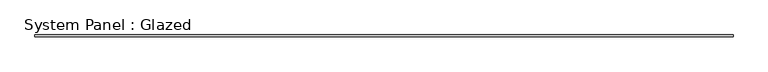
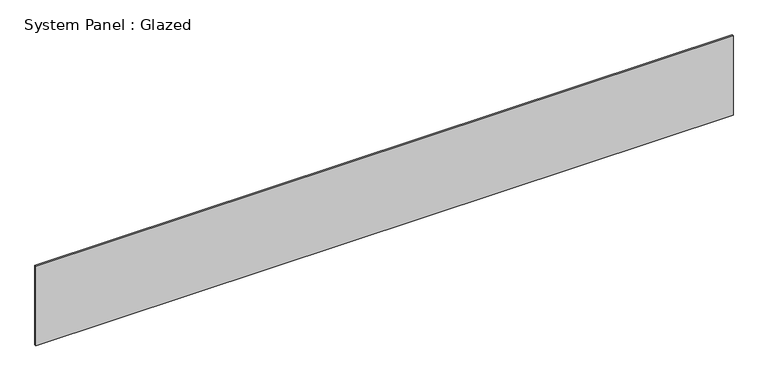
"""IFC4 building model written with IfcOpenShell, lengths in millimetres: plate geometry, System Panel : Glazed."""

from ifc_helpers import new_model, si_unit, origin, origin_with_axes, place, context, project, spatial, polyline, outline, extrude, source, transform, mapped, element, save


def system_panel_glazed_70773d7f(model_context):
    return source(origin(), model_context, "Body", "SweptSolid", [
        extrude(outline(polyline([(5054.6, 19.05), (-5054.6, 19.05), (-5054.6, 44.45), (5054.6, 44.45), (5054.6, 19.05)])), origin_with_axes(), (0.0, 0.0, 1.0), 1219.2),
    ])


if __name__ == "__main__":
    model = new_model("IFC4")
    model_context = context("Model", 3, world=origin())
    ifc_project = project(units=[si_unit("LENGTHUNIT", "METRE", prefix="MILLI")], contexts=[model_context])
    site = spatial("IfcSite", under=ifc_project)
    building = spatial("IfcBuilding", under=site)
    placement = place(None, origin())
    system_panel_glazed_shape = system_panel_glazed_70773d7f(model_context)
    element("IfcPlate", 1, ObjectType="System Panel : Glazed", at=placement, inside=building, context=model_context, shape_type="MappedRepresentation", body=[
        mapped(system_panel_glazed_shape, transform((0.0, 0.0, 0.0), x_axis=(1.0, 0.0, 0.0), y_axis=(0.0, 1.0, 0.0), z_axis=(0.0, 0.0, 1.0))),
    ])
    save(model, "model.ifc")

# Revit data of these elements
# Type "System Panel : Glazed"
#   Construction Type Id = "GSP4R"
#   Analytic Construction = "1/8 in Pilkington single glazing"
#   Visual Light Transmittance = 0.9
#   Solar Heat Gain Coefficient = 0.86
#   Heat Transfer Coefficient (U) = 1.18115 BTU/(h·ft²·°F)
# Element 1 (IfcPlate, "System Panel : Glazed")
#   Materials on its faces: "Glass"
# Materials
#   "Glass": class "Glass", colour RGB 0 128 192, transparency 0.75, Description = "Soda Lime Glass", Cost = 0
